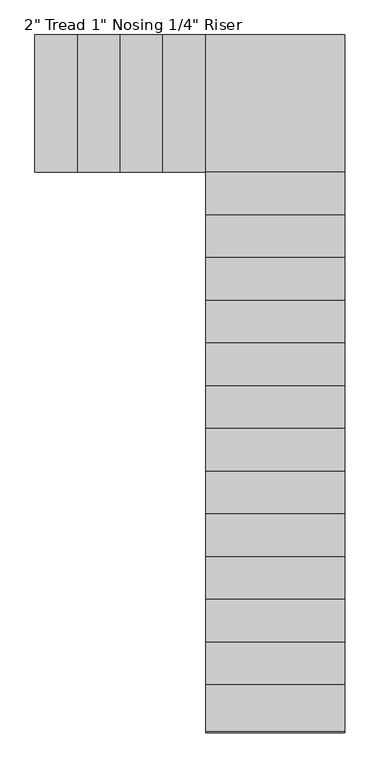
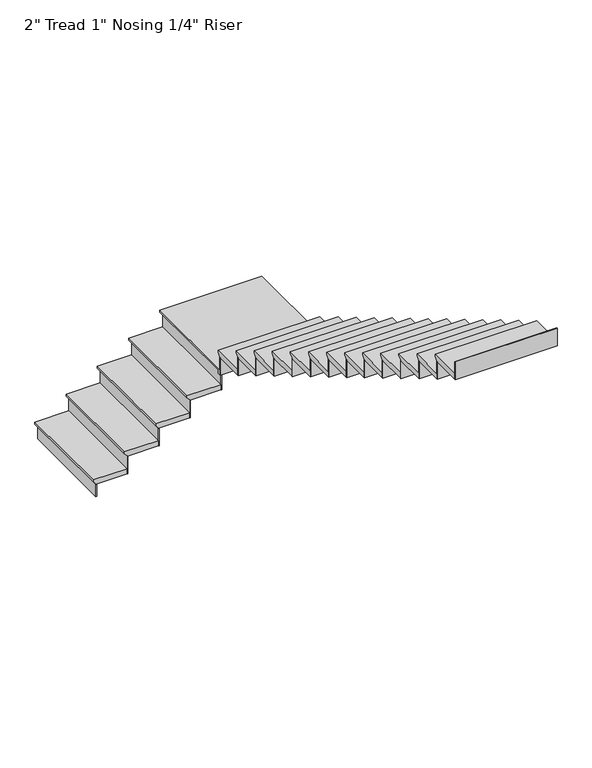
"""IFC4 building model written with IfcOpenShell, lengths in millimetres: stair flight geometry."""

from ifc_helpers import new_model, si_unit, origin, place, context, project, spatial, faceted_brep, source, transform, mapped, element, save


def stair_flight_9587ce78(model_context):
    return source(origin(), model_context, "Body", "Brep", [
        faceted_brep([(-14204.9595293, 3130.1909199, 455.0833333), (-14204.9595293, 3130.1909199, 474.1333333), (-14204.9595293, 4044.5909199, 474.1333333), (-14204.9595293, 4044.5909199, 455.0833333), (-14179.5595293, 3130.1909199, 429.6833333), (-14179.5595293, 4044.5909199, 429.6833333), (-13895.5682612, 3130.1909199, 474.1333333), (-13895.5682612, 4044.5909199, 474.1333333), (-14179.5595293, 4044.5909199, 423.3333333), (-13895.5682612, 4044.5909199, 423.3333333), (-13895.5682612, 3130.1909199, 423.3333333), (-14179.5595293, 3130.1909199, 423.3333333)], [[[0, 1, 2, 3]], [[4, 0, 3, 5]], [[2, 1, 6, 7]], [[8, 9, 10, 11]], [[2, 7, 9, 8, 5, 3]], [[8, 11, 4, 5]], [[6, 1, 0, 4, 11, 10]], [[7, 6, 10, 9]]]),
        faceted_brep([(-14179.5595293, 3130.1909199, 423.3333333), (-14179.5595293, 3130.1909199, 304.8), (-14173.2095293, 3130.1909199, 304.8), (-14173.2095293, 3130.1909199, 423.3333333), (-14179.5595293, 4044.5909199, 423.3333333), (-14173.2095293, 4044.5909199, 423.3333333), (-14173.2095293, 4044.5909199, 304.8), (-14179.5595293, 4044.5909199, 304.8)], [[[0, 1, 2, 3]], [[4, 5, 6, 7]], [[1, 0, 4, 7]], [[2, 1, 7, 6]], [[3, 2, 6, 5]], [[0, 3, 5, 4]]]),
        faceted_brep([(-13895.5682612, 3130.1909199, 592.6666667), (-13895.5682612, 3130.1909199, 423.3333333), (-13889.2182612, 3130.1909199, 423.3333333), (-13889.2182612, 3130.1909199, 592.6666667), (-13895.5682612, 4044.5909199, 592.6666667), (-13889.2182612, 4044.5909199, 592.6666667), (-13889.2182612, 4044.5909199, 423.3333333), (-13895.5682612, 4044.5909199, 423.3333333)], [[[0, 1, 2, 3]], [[4, 5, 6, 7]], [[1, 0, 4, 7]], [[2, 1, 7, 6]], [[3, 2, 6, 5]], [[0, 3, 5, 4]]]),
        faceted_brep([(-13920.9682612, 4044.5909199, 643.4666667), (-13920.9682612, 3130.1909199, 643.4666667), (-13611.576993, 3130.1909199, 643.4666667), (-13611.576993, 4044.5909199, 643.4666667), (-13895.5682612, 4044.5909199, 592.6666667), (-13611.576993, 4044.5909199, 592.6666667), (-13611.576993, 3130.1909199, 592.6666667), (-13895.5682612, 3130.1909199, 592.6666667), (-13895.5682612, 4044.5909199, 599.0166667), (-13920.9682612, 4044.5909199, 624.4166667), (-13895.5682612, 3130.1909199, 599.0166667), (-13920.9682612, 3130.1909199, 624.4166667)], [[[0, 1, 2, 3]], [[4, 5, 6, 7]], [[0, 3, 5, 4, 8, 9]], [[4, 7, 10, 8]], [[2, 1, 11, 10, 7, 6]], [[3, 2, 6, 5]], [[11, 1, 0, 9]], [[10, 11, 9, 8]]]),
        faceted_brep([(-13611.576993, 3130.1909199, 762.0), (-13611.576993, 3130.1909199, 592.6666667), (-13605.226993, 3130.1909199, 592.6666667), (-13605.226993, 3130.1909199, 762.0), (-13611.576993, 4044.5909199, 762.0), (-13605.226993, 4044.5909199, 762.0), (-13605.226993, 4044.5909199, 592.6666667), (-13611.576993, 4044.5909199, 592.6666667)], [[[0, 1, 2, 3]], [[4, 5, 6, 7]], [[1, 0, 4, 7]], [[2, 1, 7, 6]], [[3, 2, 6, 5]], [[0, 3, 5, 4]]]),
        faceted_brep([(-13636.976993, 4044.5909199, 812.8), (-13636.976993, 3130.1909199, 812.8), (-13327.5857249, 3130.1909199, 812.8), (-13327.5857249, 4044.5909199, 812.8), (-13611.576993, 4044.5909199, 762.0), (-13327.5857249, 4044.5909199, 762.0), (-13327.5857249, 3130.1909199, 762.0), (-13611.576993, 3130.1909199, 762.0), (-13611.576993, 4044.5909199, 768.35), (-13636.976993, 4044.5909199, 793.75), (-13611.576993, 3130.1909199, 768.35), (-13636.976993, 3130.1909199, 793.75)], [[[0, 1, 2, 3]], [[4, 5, 6, 7]], [[0, 3, 5, 4, 8, 9]], [[4, 7, 10, 8]], [[2, 1, 11, 10, 7, 6]], [[3, 2, 6, 5]], [[11, 1, 0, 9]], [[10, 11, 9, 8]]]),
        faceted_brep([(-13327.5857249, 3130.1909199, 931.3333333), (-13327.5857249, 3130.1909199, 762.0), (-13321.2357249, 3130.1909199, 762.0), (-13321.2357249, 3130.1909199, 931.3333333), (-13327.5857249, 4044.5909199, 931.3333333), (-13321.2357249, 4044.5909199, 931.3333333), (-13321.2357249, 4044.5909199, 762.0), (-13327.5857249, 4044.5909199, 762.0)], [[[0, 1, 2, 3]], [[4, 5, 6, 7]], [[1, 0, 4, 7]], [[2, 1, 7, 6]], [[3, 2, 6, 5]], [[0, 3, 5, 4]]]),
        faceted_brep([(-13352.9857249, 4044.5909199, 982.1333333), (-13352.9857249, 3130.1909199, 982.1333333), (-13043.5007021, 3130.1909199, 982.1333333), (-13043.5007021, 4044.5909199, 982.1333333), (-13327.5857249, 4044.5909199, 931.3333333), (-13043.5007021, 4044.5909199, 931.3333333), (-13043.5007021, 3130.1909199, 931.3333333), (-13327.5857249, 3130.1909199, 931.3333333), (-13327.5857249, 4044.5909199, 937.6833333), (-13352.9857249, 4044.5909199, 963.0833333), (-13327.5857249, 3130.1909199, 937.6833333), (-13352.9857249, 3130.1909199, 963.0833333)], [[[0, 1, 2, 3]], [[4, 5, 6, 7]], [[0, 3, 5, 4, 8, 9]], [[4, 7, 10, 8]], [[2, 1, 11, 10, 7, 6]], [[3, 2, 6, 5]], [[11, 1, 0, 9]], [[10, 11, 9, 8]]]),
        faceted_brep([(-13043.5007021, 3130.1909199, 1100.6666667), (-13043.5007021, 3130.1909199, 931.3333333), (-13037.1507021, 3130.1909199, 931.3333333), (-13037.1507021, 3130.1909199, 1100.6666667), (-13043.5007021, 4044.5909199, 1100.6666667), (-13037.1507021, 4044.5909199, 1100.6666667), (-13037.1507021, 4044.5909199, 931.3333333), (-13043.5007021, 4044.5909199, 931.3333333)], [[[0, 1, 2, 3]], [[4, 5, 6, 7]], [[1, 0, 4, 7]], [[2, 1, 7, 6]], [[3, 2, 6, 5]], [[0, 3, 5, 4]]]),
        faceted_brep([(-12143.6860997, 3104.7909199, 1151.4666667), (-12143.6860997, 4044.5909199, 1151.4666667), (-13068.9007021, 4044.5909199, 1151.4666667), (-13068.9007021, 3104.7909199, 1151.4666667), (-12143.6860997, 4044.5909199, 1100.6666667), (-12143.6860997, 3104.7909199, 1100.6666667), (-13068.9007021, 3104.7909199, 1100.6666667), (-13068.9007021, 3130.1909199, 1100.6666667), (-13043.5007021, 3130.1909199, 1100.6666667), (-13043.5007021, 4044.5909199, 1100.6666667), (-13043.5007021, 4044.5909199, 1107.0166667), (-13068.9007021, 4044.5909199, 1132.4166667), (-13043.5007021, 3130.1909199, 1107.0166667), (-13068.9007021, 3130.1909199, 1132.4166667)], [[[0, 1, 2, 3]], [[4, 5, 6, 7, 8, 9]], [[1, 0, 5, 4]], [[2, 1, 4, 9, 10, 11]], [[9, 8, 12, 10]], [[8, 7, 13, 12]], [[3, 2, 11, 13, 7, 6]], [[0, 3, 6, 5]], [[11, 10, 12, 13]]]),
        faceted_brep([(-13068.9007021, 3104.7909199, 1270.0), (-13068.9007021, 3104.7909199, 1100.6666667), (-13068.9007021, 3098.4409199, 1100.6666667), (-13068.9007021, 3098.4409199, 1270.0), (-12143.6860997, 3104.7909199, 1270.0), (-12143.6860997, 3098.4409199, 1270.0), (-12143.6860997, 3098.4409199, 1100.6666667), (-12143.6860997, 3104.7909199, 1100.6666667)], [[[0, 1, 2, 3]], [[4, 5, 6, 7]], [[1, 0, 4, 7]], [[2, 1, 7, 6]], [[3, 2, 6, 5]], [[0, 3, 5, 4]]]),
        faceted_brep([(-12143.6860997, 3130.1909199, 1320.8), (-13068.9007021, 3130.1909199, 1320.8), (-13068.9007021, 2820.3109199, 1320.8), (-12143.6860997, 2820.3109199, 1320.8), (-12143.6860997, 3104.7909199, 1270.0), (-12143.6860997, 2820.3109199, 1270.0), (-13068.9007021, 2820.3109199, 1270.0), (-13068.9007021, 3104.7909199, 1270.0), (-12143.6860997, 3104.7909199, 1276.35), (-12143.6860997, 3130.1909199, 1301.75), (-13068.9007021, 3104.7909199, 1276.35), (-13068.9007021, 3130.1909199, 1301.75)], [[[0, 1, 2, 3]], [[4, 5, 6, 7]], [[0, 3, 5, 4, 8, 9]], [[4, 7, 10, 8]], [[2, 1, 11, 10, 7, 6]], [[3, 2, 6, 5]], [[11, 1, 0, 9]], [[10, 11, 9, 8]]]),
        faceted_brep([(-13068.9007021, 2820.3109199, 1439.3333333), (-13068.9007021, 2820.3109199, 1270.0), (-13068.9007021, 2813.9609199, 1270.0), (-13068.9007021, 2813.9609199, 1439.3333333), (-12143.6860997, 2820.3109199, 1439.3333333), (-12143.6860997, 2813.9609199, 1439.3333333), (-12143.6860997, 2813.9609199, 1270.0), (-12143.6860997, 2820.3109199, 1270.0)], [[[0, 1, 2, 3]], [[4, 5, 6, 7]], [[1, 0, 4, 7]], [[2, 1, 7, 6]], [[3, 2, 6, 5]], [[0, 3, 5, 4]]]),
        faceted_brep([(-12143.6860997, 2845.7109199, 1490.1333333), (-13068.9007021, 2845.7109199, 1490.1333333), (-13068.9007021, 2535.8309199, 1490.1333333), (-12143.6860997, 2535.8309199, 1490.1333333), (-12143.6860997, 2820.3109199, 1439.3333333), (-12143.6860997, 2535.8309199, 1439.3333333), (-13068.9007021, 2535.8309199, 1439.3333333), (-13068.9007021, 2820.3109199, 1439.3333333), (-12143.6860997, 2820.3109199, 1445.6833333), (-12143.6860997, 2845.7109199, 1471.0833333), (-13068.9007021, 2820.3109199, 1445.6833333), (-13068.9007021, 2845.7109199, 1471.0833333)], [[[0, 1, 2, 3]], [[4, 5, 6, 7]], [[0, 3, 5, 4, 8, 9]], [[4, 7, 10, 8]], [[2, 1, 11, 10, 7, 6]], [[3, 2, 6, 5]], [[11, 1, 0, 9]], [[10, 11, 9, 8]]]),
        faceted_brep([(-13068.9007021, 2535.8309199, 1608.6666667), (-13068.9007021, 2535.8309199, 1439.3333333), (-13068.9007021, 2529.4809199, 1439.3333333), (-13068.9007021, 2529.4809199, 1608.6666667), (-12143.6860997, 2535.8309199, 1608.6666667), (-12143.6860997, 2529.4809199, 1608.6666667), (-12143.6860997, 2529.4809199, 1439.3333333), (-12143.6860997, 2535.8309199, 1439.3333333)], [[[0, 1, 2, 3]], [[4, 5, 6, 7]], [[1, 0, 4, 7]], [[2, 1, 7, 6]], [[3, 2, 6, 5]], [[0, 3, 5, 4]]]),
        faceted_brep([(-12143.6860997, 2561.2309199, 1659.4666667), (-13068.9007021, 2561.2309199, 1659.4666667), (-13068.9007021, 2251.3509199, 1659.4666667), (-12143.6860997, 2251.3509199, 1659.4666667), (-12143.6860997, 2535.8309199, 1608.6666667), (-12143.6860997, 2251.3509199, 1608.6666667), (-13068.9007021, 2251.3509199, 1608.6666667), (-13068.9007021, 2535.8309199, 1608.6666667), (-12143.6860997, 2535.8309199, 1615.0166667), (-12143.6860997, 2561.2309199, 1640.4166667), (-13068.9007021, 2535.8309199, 1615.0166667), (-13068.9007021, 2561.2309199, 1640.4166667)], [[[0, 1, 2, 3]], [[4, 5, 6, 7]], [[0, 3, 5, 4, 8, 9]], [[4, 7, 10, 8]], [[2, 1, 11, 10, 7, 6]], [[3, 2, 6, 5]], [[11, 1, 0, 9]], [[10, 11, 9, 8]]]),
        faceted_brep([(-13068.9007021, 2251.3509199, 1778.0), (-13068.9007021, 2251.3509199, 1608.6666667), (-13068.9007021, 2245.0009199, 1608.6666667), (-13068.9007021, 2245.0009199, 1778.0), (-12143.6860997, 2251.3509199, 1778.0), (-12143.6860997, 2245.0009199, 1778.0), (-12143.6860997, 2245.0009199, 1608.6666667), (-12143.6860997, 2251.3509199, 1608.6666667)], [[[0, 1, 2, 3]], [[4, 5, 6, 7]], [[1, 0, 4, 7]], [[2, 1, 7, 6]], [[3, 2, 6, 5]], [[0, 3, 5, 4]]]),
        faceted_brep([(-12143.6860997, 2276.7509199, 1828.8), (-13068.9007021, 2276.7509199, 1828.8), (-13068.9007021, 1966.8709199, 1828.8), (-12143.6860997, 1966.8709199, 1828.8), (-12143.6860997, 2251.3509199, 1778.0), (-12143.6860997, 1966.8709199, 1778.0), (-13068.9007021, 1966.8709199, 1778.0), (-13068.9007021, 2251.3509199, 1778.0), (-12143.6860997, 2251.3509199, 1784.35), (-12143.6860997, 2276.7509199, 1809.75), (-13068.9007021, 2251.3509199, 1784.35), (-13068.9007021, 2276.7509199, 1809.75)], [[[0, 1, 2, 3]], [[4, 5, 6, 7]], [[0, 3, 5, 4, 8, 9]], [[4, 7, 10, 8]], [[2, 1, 11, 10, 7, 6]], [[3, 2, 6, 5]], [[11, 1, 0, 9]], [[10, 11, 9, 8]]]),
        faceted_brep([(-13068.9007021, 1966.8709199, 1947.3333333), (-13068.9007021, 1966.8709199, 1778.0), (-13068.9007021, 1960.5209199, 1778.0), (-13068.9007021, 1960.5209199, 1947.3333333), (-12143.6860997, 1966.8709199, 1947.3333333), (-12143.6860997, 1960.5209199, 1947.3333333), (-12143.6860997, 1960.5209199, 1778.0), (-12143.6860997, 1966.8709199, 1778.0)], [[[0, 1, 2, 3]], [[4, 5, 6, 7]], [[1, 0, 4, 7]], [[2, 1, 7, 6]], [[3, 2, 6, 5]], [[0, 3, 5, 4]]]),
        faceted_brep([(-12143.6860997, 1992.2709199, 1998.1333333), (-13068.9007021, 1992.2709199, 1998.1333333), (-13068.9007021, 1682.3909199, 1998.1333333), (-12143.6860997, 1682.3909199, 1998.1333333), (-12143.6860997, 1966.8709199, 1947.3333333), (-12143.6860997, 1682.3909199, 1947.3333333), (-13068.9007021, 1682.3909199, 1947.3333333), (-13068.9007021, 1966.8709199, 1947.3333333), (-12143.6860997, 1966.8709199, 1953.6833333), (-12143.6860997, 1992.2709199, 1979.0833333), (-13068.9007021, 1966.8709199, 1953.6833333), (-13068.9007021, 1992.2709199, 1979.0833333)], [[[0, 1, 2, 3]], [[4, 5, 6, 7]], [[0, 3, 5, 4, 8, 9]], [[4, 7, 10, 8]], [[2, 1, 11, 10, 7, 6]], [[3, 2, 6, 5]], [[11, 1, 0, 9]], [[10, 11, 9, 8]]]),
        faceted_brep([(-13068.9007021, 1682.3909199, 2116.6666667), (-13068.9007021, 1682.3909199, 1947.3333333), (-13068.9007021, 1676.0409199, 1947.3333333), (-13068.9007021, 1676.0409199, 2116.6666667), (-12143.6860997, 1682.3909199, 2116.6666667), (-12143.6860997, 1676.0409199, 2116.6666667), (-12143.6860997, 1676.0409199, 1947.3333333), (-12143.6860997, 1682.3909199, 1947.3333333)], [[[0, 1, 2, 3]], [[4, 5, 6, 7]], [[1, 0, 4, 7]], [[2, 1, 7, 6]], [[3, 2, 6, 5]], [[0, 3, 5, 4]]]),
        faceted_brep([(-12143.6860997, 1707.7909199, 2167.4666667), (-13068.9007021, 1707.7909199, 2167.4666667), (-13068.9007021, 1397.9109198, 2167.4666667), (-12143.6860997, 1397.9109198, 2167.4666667), (-12143.6860997, 1682.3909199, 2116.6666667), (-12143.6860997, 1397.9109198, 2116.6666667), (-13068.9007021, 1397.9109198, 2116.6666667), (-13068.9007021, 1682.3909199, 2116.6666667), (-12143.6860997, 1682.3909199, 2123.0166667), (-12143.6860997, 1707.7909199, 2148.4166667), (-13068.9007021, 1682.3909199, 2123.0166667), (-13068.9007021, 1707.7909199, 2148.4166667)], [[[0, 1, 2, 3]], [[4, 5, 6, 7]], [[0, 3, 5, 4, 8, 9]], [[4, 7, 10, 8]], [[2, 1, 11, 10, 7, 6]], [[3, 2, 6, 5]], [[11, 1, 0, 9]], [[10, 11, 9, 8]]]),
        faceted_brep([(-13068.9007021, 1397.9109199, 2286.0), (-13068.9007021, 1397.9109199, 2116.6666667), (-13068.9007021, 1391.5609199, 2116.6666667), (-13068.9007021, 1391.5609199, 2286.0), (-12143.6860997, 1397.9109199, 2286.0), (-12143.6860997, 1391.5609199, 2286.0), (-12143.6860997, 1391.5609199, 2116.6666667), (-12143.6860997, 1397.9109199, 2116.6666667)], [[[0, 1, 2, 3]], [[4, 5, 6, 7]], [[1, 0, 4, 7]], [[2, 1, 7, 6]], [[3, 2, 6, 5]], [[0, 3, 5, 4]]]),
        faceted_brep([(-12143.6860997, 1423.3109199, 2336.8), (-13068.9007021, 1423.3109199, 2336.8), (-13068.9007021, 1113.4309198, 2336.8), (-12143.6860997, 1113.4309198, 2336.8), (-12143.6860997, 1397.9109199, 2286.0), (-12143.6860997, 1113.4309198, 2286.0), (-13068.9007021, 1113.4309198, 2286.0), (-13068.9007021, 1397.9109199, 2286.0), (-12143.6860997, 1397.9109199, 2292.35), (-12143.6860997, 1423.3109199, 2317.75), (-13068.9007021, 1397.9109199, 2292.35), (-13068.9007021, 1423.3109199, 2317.75)], [[[0, 1, 2, 3]], [[4, 5, 6, 7]], [[0, 3, 5, 4, 8, 9]], [[4, 7, 10, 8]], [[2, 1, 11, 10, 7, 6]], [[3, 2, 6, 5]], [[11, 1, 0, 9]], [[10, 11, 9, 8]]]),
        faceted_brep([(-13068.9007021, 1113.4309199, 2455.3333333), (-13068.9007021, 1113.4309199, 2286.0), (-13068.9007021, 1107.0809199, 2286.0), (-13068.9007021, 1107.0809199, 2455.3333333), (-12143.6860997, 1113.4309199, 2455.3333333), (-12143.6860997, 1107.0809199, 2455.3333333), (-12143.6860997, 1107.0809199, 2286.0), (-12143.6860997, 1113.4309199, 2286.0)], [[[0, 1, 2, 3]], [[4, 5, 6, 7]], [[1, 0, 4, 7]], [[2, 1, 7, 6]], [[3, 2, 6, 5]], [[0, 3, 5, 4]]]),
        faceted_brep([(-12143.6860997, 1138.8309199, 2506.1333333), (-13068.9007021, 1138.8309199, 2506.1333333), (-13068.9007021, 828.9509198, 2506.1333333), (-12143.6860997, 828.9509198, 2506.1333333), (-12143.6860997, 1113.4309199, 2455.3333333), (-12143.6860997, 828.9509198, 2455.3333333), (-13068.9007021, 828.9509198, 2455.3333333), (-13068.9007021, 1113.4309199, 2455.3333333), (-12143.6860997, 1113.4309199, 2461.6833333), (-12143.6860997, 1138.8309199, 2487.0833333), (-13068.9007021, 1113.4309199, 2461.6833333), (-13068.9007021, 1138.8309199, 2487.0833333)], [[[0, 1, 2, 3]], [[4, 5, 6, 7]], [[0, 3, 5, 4, 8, 9]], [[4, 7, 10, 8]], [[2, 1, 11, 10, 7, 6]], [[3, 2, 6, 5]], [[11, 1, 0, 9]], [[10, 11, 9, 8]]]),
        faceted_brep([(-13068.9007021, 828.9509199, 2624.6666667), (-13068.9007021, 828.9509199, 2455.3333333), (-13068.9007021, 822.6009199, 2455.3333333), (-13068.9007021, 822.6009199, 2624.6666667), (-12143.6860997, 828.9509199, 2624.6666667), (-12143.6860997, 822.6009199, 2624.6666667), (-12143.6860997, 822.6009199, 2455.3333333), (-12143.6860997, 828.9509199, 2455.3333333)], [[[0, 1, 2, 3]], [[4, 5, 6, 7]], [[1, 0, 4, 7]], [[2, 1, 7, 6]], [[3, 2, 6, 5]], [[0, 3, 5, 4]]]),
        faceted_brep([(-12143.6860997, 854.3509199, 2675.4666667), (-13068.9007021, 854.3509199, 2675.4666667), (-13068.9007021, 544.4709198, 2675.4666667), (-12143.6860997, 544.4709198, 2675.4666667), (-12143.6860997, 828.9509199, 2624.6666667), (-12143.6860997, 544.4709198, 2624.6666667), (-13068.9007021, 544.4709198, 2624.6666667), (-13068.9007021, 828.9509199, 2624.6666667), (-12143.6860997, 828.9509199, 2631.0166667), (-12143.6860997, 854.3509199, 2656.4166667), (-13068.9007021, 828.9509199, 2631.0166667), (-13068.9007021, 854.3509199, 2656.4166667)], [[[0, 1, 2, 3]], [[4, 5, 6, 7]], [[0, 3, 5, 4, 8, 9]], [[4, 7, 10, 8]], [[2, 1, 11, 10, 7, 6]], [[3, 2, 6, 5]], [[11, 1, 0, 9]], [[10, 11, 9, 8]]]),
        faceted_brep([(-13068.9007021, 544.4709198, 2794.0), (-13068.9007021, 544.4709198, 2624.6666667), (-13068.9007021, 538.1209198, 2624.6666667), (-13068.9007021, 538.1209198, 2794.0), (-12143.6860997, 544.4709198, 2794.0), (-12143.6860997, 538.1209198, 2794.0), (-12143.6860997, 538.1209198, 2624.6666667), (-12143.6860997, 544.4709198, 2624.6666667)], [[[0, 1, 2, 3]], [[4, 5, 6, 7]], [[1, 0, 4, 7]], [[2, 1, 7, 6]], [[3, 2, 6, 5]], [[0, 3, 5, 4]]]),
        faceted_brep([(-12143.6860997, 569.8709198, 2844.8), (-13068.9007021, 569.8709198, 2844.8), (-13068.9007021, 260.0107636, 2844.8), (-12143.6860997, 260.0107636, 2844.8), (-12143.6860997, 544.4709198, 2794.0), (-12143.6860997, 260.0107636, 2794.0), (-13068.9007021, 260.0107636, 2794.0), (-13068.9007021, 544.4709198, 2794.0), (-12143.6860997, 544.4709198, 2800.35), (-12143.6860997, 569.8709198, 2825.75), (-13068.9007021, 544.4709198, 2800.35), (-13068.9007021, 569.8709198, 2825.75)], [[[0, 1, 2, 3]], [[4, 5, 6, 7]], [[0, 3, 5, 4, 8, 9]], [[4, 7, 10, 8]], [[2, 1, 11, 10, 7, 6]], [[3, 2, 6, 5]], [[11, 1, 0, 9]], [[10, 11, 9, 8]]]),
        faceted_brep([(-13068.9007021, 260.0107636, 2963.3333333), (-13068.9007021, 260.0107636, 2794.0), (-13068.9007021, 253.6607636, 2794.0), (-13068.9007021, 253.6607636, 2963.3333333), (-12143.6860997, 260.0107636, 2963.3333333), (-12143.6860997, 253.6607636, 2963.3333333), (-12143.6860997, 253.6607636, 2794.0), (-12143.6860997, 260.0107636, 2794.0)], [[[0, 1, 2, 3]], [[4, 5, 6, 7]], [[1, 0, 4, 7]], [[2, 1, 7, 6]], [[3, 2, 6, 5]], [[0, 3, 5, 4]]]),
        faceted_brep([(-12143.6860997, 285.4107636, 3014.1333333), (-13068.9007021, 285.4107636, 3014.1333333), (-13068.9007021, -24.4493927, 3014.1333333), (-12143.6860997, -24.4493927, 3014.1333333), (-12143.6860997, 260.0107636, 2963.3333333), (-12143.6860997, -24.4493927, 2963.3333333), (-13068.9007021, -24.4493927, 2963.3333333), (-13068.9007021, 260.0107636, 2963.3333333), (-12143.6860997, 260.0107636, 2969.6833333), (-12143.6860997, 285.4107636, 2995.0833333), (-13068.9007021, 260.0107636, 2969.6833333), (-13068.9007021, 285.4107636, 2995.0833333)], [[[0, 1, 2, 3]], [[4, 5, 6, 7]], [[0, 3, 5, 4, 8, 9]], [[4, 7, 10, 8]], [[2, 1, 11, 10, 7, 6]], [[3, 2, 6, 5]], [[11, 1, 0, 9]], [[10, 11, 9, 8]]]),
        faceted_brep([(-13068.9007021, -24.4493927, 3132.6666667), (-13068.9007021, -24.4493927, 2963.3333333), (-13068.9007021, -30.7993927, 2963.3333333), (-13068.9007021, -30.7993927, 3132.6666667), (-12143.6860997, -24.4493927, 3132.6666667), (-12143.6860997, -30.7993927, 3132.6666667), (-12143.6860997, -30.7993927, 2963.3333333), (-12143.6860997, -24.4493927, 2963.3333333)], [[[0, 1, 2, 3]], [[4, 5, 6, 7]], [[1, 0, 4, 7]], [[2, 1, 7, 6]], [[3, 2, 6, 5]], [[0, 3, 5, 4]]]),
        faceted_brep([(-12143.6860997, 0.9506073, 3183.4666667), (-13068.9007021, 0.9506073, 3183.4666667), (-13068.9007021, -308.9095489, 3183.4666667), (-12143.6860997, -308.9095489, 3183.4666667), (-12143.6860997, -24.4493927, 3132.6666667), (-12143.6860997, -308.9095489, 3132.6666667), (-13068.9007021, -308.9095489, 3132.6666667), (-13068.9007021, -24.4493927, 3132.6666667), (-12143.6860997, -24.4493927, 3139.0166667), (-12143.6860997, 0.9506073, 3164.4166667), (-13068.9007021, -24.4493927, 3139.0166667), (-13068.9007021, 0.9506073, 3164.4166667)], [[[0, 1, 2, 3]], [[4, 5, 6, 7]], [[0, 3, 5, 4, 8, 9]], [[4, 7, 10, 8]], [[2, 1, 11, 10, 7, 6]], [[3, 2, 6, 5]], [[11, 1, 0, 9]], [[10, 11, 9, 8]]]),
        faceted_brep([(-13068.9007021, -308.9095489, 3302.0), (-13068.9007021, -308.9095489, 3132.6666667), (-13068.9007021, -315.2595489, 3132.6666667), (-13068.9007021, -315.2595489, 3302.0), (-12143.6860997, -308.9095489, 3302.0), (-12143.6860997, -315.2595489, 3302.0), (-12143.6860997, -315.2595489, 3132.6666667), (-12143.6860997, -308.9095489, 3132.6666667)], [[[0, 1, 2, 3]], [[4, 5, 6, 7]], [[1, 0, 4, 7]], [[2, 1, 7, 6]], [[3, 2, 6, 5]], [[0, 3, 5, 4]]]),
        faceted_brep([(-13068.9007021, -593.3697052, 3471.3333333), (-13068.9007021, -593.3697052, 3302.0), (-13068.9007021, -599.7197052, 3302.0), (-13068.9007021, -599.7197052, 3471.3333333), (-12143.6860997, -593.3697052, 3471.3333333), (-12143.6860997, -599.7197052, 3471.3333333), (-12143.6860997, -599.7197052, 3302.0), (-12143.6860997, -593.3697052, 3302.0)], [[[0, 1, 2, 3]], [[4, 5, 6, 7]], [[1, 0, 4, 7]], [[2, 1, 7, 6]], [[3, 2, 6, 5]], [[0, 3, 5, 4]]]),
        faceted_brep([(-12143.6860997, -283.5095489, 3352.8), (-13068.9007021, -283.5095489, 3352.8), (-13068.9007021, -593.3697052, 3352.8), (-12143.6860997, -593.3697052, 3352.8), (-12143.6860997, -308.9095489, 3302.0), (-12143.6860997, -593.3697052, 3302.0), (-13068.9007021, -593.3697052, 3302.0), (-13068.9007021, -308.9095489, 3302.0), (-12143.6860997, -308.9095489, 3308.35), (-12143.6860997, -283.5095489, 3333.75), (-13068.9007021, -308.9095489, 3308.35), (-13068.9007021, -283.5095489, 3333.75)], [[[0, 1, 2, 3]], [[4, 5, 6, 7]], [[0, 3, 5, 4, 8, 9]], [[4, 7, 10, 8]], [[2, 1, 11, 10, 7, 6]], [[3, 2, 6, 5]], [[11, 1, 0, 9]], [[10, 11, 9, 8]]]),
    ])


if __name__ == "__main__":
    model = new_model("IFC4")
    model_context = context("Model", 3, world=origin())
    ifc_project = project(units=[si_unit("LENGTHUNIT", "METRE", prefix="MILLI")], contexts=[model_context])
    site = spatial("IfcSite", under=ifc_project)
    building = spatial("IfcBuilding", under=site)
    placement = place(None, origin())
    stair_flight_shape = stair_flight_9587ce78(model_context)
    element("IfcStairFlight", 1, ObjectType="2\" Tread 1\" Nosing 1/4\" Riser", at=placement, inside=building, context=model_context, shape_type="MappedRepresentation", body=[
        mapped(stair_flight_shape, transform((0.0, 0.0, 0.0), x_axis=(1.0, 0.0, 0.0), y_axis=(0.0, 1.0, 0.0), z_axis=(0.0, 0.0, 1.0))),
    ])
    save(model, "model.ifc")
